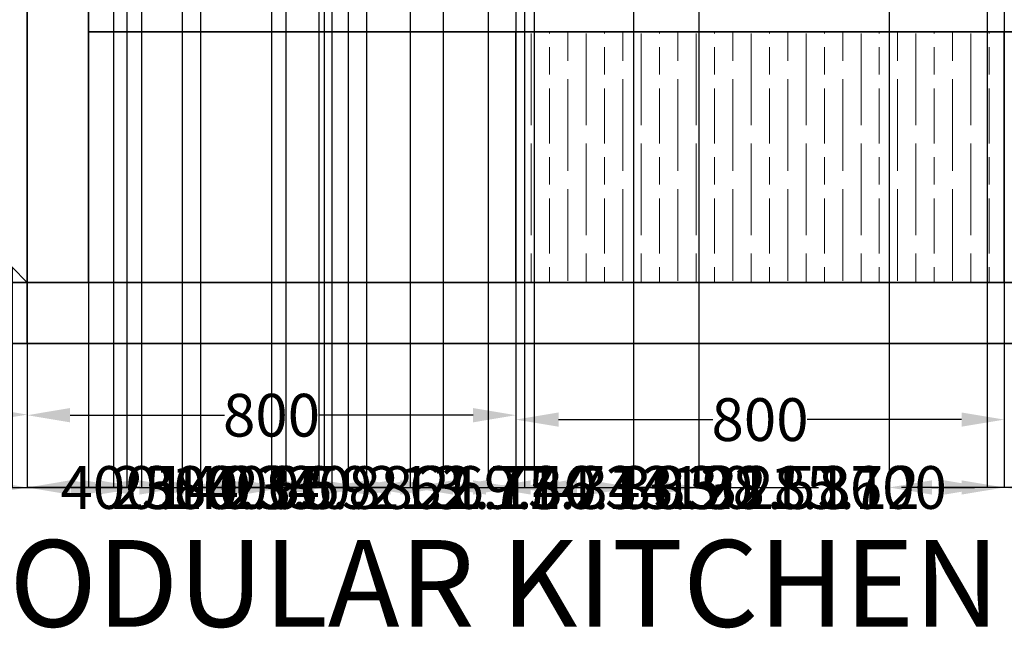
# Model space of a CAD drawing. Units: inches. Extents: x 600 to 5582, y -464 to 3142.
# Tile 2 of 9: x 1772 to 3385, y -464 to 532. Entities that reach past the tile are written whole.
import ezdxf

# ---------------------------------------------------------------- set-up
doc = ezdxf.new("R2010")
doc.units = ezdxf.units.IN
doc.header["$MEASUREMENT"] = 0
for name, color, linetype, lineweight in [('A-ANNO-DIMS', 2, 'Continuous', 18), ('A-ANNO-TEXT', 7, 'Continuous', 25), ('A-ELEV', 7, 'Continuous', 35), ('A-ELEV-PATT', 252, 'Continuous', 13)]:
    doc.layers.add(name, color=color, linetype=linetype, lineweight=lineweight)
doc.styles.get("Standard").update_dxf_attribs({"font": 'arial.ttf'})
doc.dimstyles.get("Standard").update_dxf_attribs({"dimtxt": 70, "dimasz": 70, "dimexe": 0.18, "dimexo": 0.0625, "dimgap": 0.09, "dimtad": 0, "dimtih": 1, "dimtoh": 1, "dimdec": 0, "dimzin": 0, "dimdsep": 46, "dimtxsty": 'Standard', "dimcen": 0.09, "dimadec": 0, "dimazin": 0, "dimtfac": 1, "dimtdec": 0, "dimtofl": 0, "dimtmove": 0, "dimatfit": 3, "dimfxl": 1, "dimtolj": 1, "dimtzin": 0, "dimarcsym": 0})

# ---------------------------------------------------------------- blocks, each defined once
blk = doc.blocks.new('*D10')
at = {"layer": 'A-ANNO-DIMS', "color": 0, "lineweight": -2, "transparency": 16777216}
for p, q in [((1384.7, 2.4), (1384.7, -113.9)), ((1784.7, 2.4), (1784.7, -113.9)), ((1454.7, -113.8), (1506, -113.8)), ((1714.7, -113.8), (1663.5, -113.8))]:
    blk.add_line(p, q, dxfattribs=at)
at = {"layer": 'A-ANNO-DIMS', "color": 0, "transparency": 16777216}
for points in [[(1454.7, -102.1), (1454.7, -125.4), (1384.7, -113.8)], [(1714.7, -102.1), (1714.7, -125.4), (1784.7, -113.8)]]:
    blk.add_solid(points, dxfattribs=at)
at = {"layer": 'Defpoints', "color": 0, "transparency": 16777216}
for p in [(1384.7, 2.4), (1784.7, 2.4), (1784.7, -113.8)]:
    blk.add_point(p, dxfattribs=at)
at = {"layer": 'A-ANNO-DIMS', "color": 0, "transparency": 16777216, "insert": (1584.7, -113.8), "char_height": 70, "attachment_point": 5}
blk.add_mtext('\\A1;400', dxfattribs=at)
blk = doc.blocks.new('*D11')
at = {"layer": 'A-ANNO-DIMS', "color": 0, "lineweight": -2, "transparency": 16777216}
for p, q in [((1784.7, 2.4), (1784.7, -115)), ((2584.7, 2.4), (2584.7, -115)), ((1854.7, -114.8), (2107.4, -114.8)), ((2514.7, -114.8), (2262.1, -114.8))]:
    blk.add_line(p, q, dxfattribs=at)
at = {"layer": 'A-ANNO-DIMS', "color": 0, "transparency": 16777216}
for points in [[(1854.7, -103.1), (1854.7, -126.5), (1784.7, -114.8)], [(2514.7, -103.1), (2514.7, -126.5), (2584.7, -114.8)]]:
    blk.add_solid(points, dxfattribs=at)
at = {"layer": 'Defpoints', "color": 0, "transparency": 16777216}
for p in [(1784.7, 2.4), (2584.7, 2.4), (2584.7, -114.8)]:
    blk.add_point(p, dxfattribs=at)
at = {"layer": 'A-ANNO-DIMS', "color": 0, "transparency": 16777216, "insert": (2184.7, -114.8), "char_height": 70, "attachment_point": 5}
blk.add_mtext('\\A1;800', dxfattribs=at)
blk = doc.blocks.new('*D12')
at = {"layer": 'A-ANNO-DIMS', "color": 0, "lineweight": -2, "transparency": 16777216}
for p, q in [((2584.7, 2.4), (2584.7, -122.1)), ((3384.7, 2.4), (3384.7, -122.1)), ((2654.7, -122), (2907.4, -122)), ((3314.7, -122), (3062.1, -122))]:
    blk.add_line(p, q, dxfattribs=at)
at = {"layer": 'A-ANNO-DIMS', "color": 0, "transparency": 16777216}
for points in [[(2654.7, -110.3), (2654.7, -133.6), (2584.7, -122)], [(3314.7, -110.3), (3314.7, -133.6), (3384.7, -122)]]:
    blk.add_solid(points, dxfattribs=at)
at = {"layer": 'Defpoints', "color": 0, "transparency": 16777216}
for p in [(2584.7, 2.4), (3384.7, 2.4), (3384.7, -122)]:
    blk.add_point(p, dxfattribs=at)
at = {"layer": 'A-ANNO-DIMS', "color": 0, "transparency": 16777216, "insert": (2984.7, -122), "char_height": 70, "attachment_point": 5}
blk.add_mtext('\\A1;800', dxfattribs=at)
blk = doc.blocks.new('*D21')
at = {"layer": 'A-ANNO-DIMS', "color": 0, "lineweight": -2, "transparency": 16777216}
for p, q in [((1384.7, 2.4), (1384.7, -233.3)), ((4984.7, 2.4), (4984.7, -233.3)), ((1454.7, -233.1), (3080.3, -233.1)), ((4914.7, -233.1), (3289.2, -233.1))]:
    blk.add_line(p, q, dxfattribs=at)
at = {"layer": 'A-ANNO-DIMS', "color": 0, "transparency": 16777216}
for points in [[(1454.7, -221.4), (1454.7, -244.7), (1384.7, -233.1)], [(4914.7, -221.4), (4914.7, -244.7), (4984.7, -233.1)]]:
    blk.add_solid(points, dxfattribs=at)
at = {"layer": 'Defpoints', "color": 0, "transparency": 16777216}
for p in [(1384.7, 2.4), (4984.7, 2.4), (4984.7, -233.1)]:
    blk.add_point(p, dxfattribs=at)
at = {"layer": 'A-ANNO-DIMS', "color": 0, "transparency": 16777216, "insert": (3184.7, -233.1), "char_height": 70, "attachment_point": 5}
blk.add_mtext('\\A1;3600', dxfattribs=at)
blk = doc.blocks.new('*D25')
at = {"layer": 'A-ANNO-DIMS', "color": 0, "lineweight": -2, "transparency": 16777216}
for p, q in [((2584.7, 1680.8), (2584.7, -233.3)), ((2615, 1655.8), (2615, -233.3)), ((2514.7, -233.1), (2444.7, -233.1)), ((2685, -233.1), (2755, -233.1))]:
    blk.add_line(p, q, dxfattribs=at)
at = {"layer": 'A-ANNO-DIMS', "color": 0, "transparency": 16777216}
for points in [[(2514.7, -221.4), (2514.7, -244.7), (2584.7, -233.1)], [(2685, -221.4), (2685, -244.7), (2615, -233.1)]]:
    blk.add_solid(points, dxfattribs=at)
at = {"layer": 'Defpoints', "color": 0, "transparency": 16777216}
for p in [(2584.7, 1680.8), (2615, 1655.8), (2615, -233.1)]:
    blk.add_point(p, dxfattribs=at)
at = {"layer": 'A-ANNO-DIMS', "color": 0, "transparency": 16777216, "insert": (2873.3, -233.1), "char_height": 70, "attachment_point": 5}
blk.add_mtext('\\A1;30.28', dxfattribs=at)
blk = doc.blocks.new('*D26')
at = {"layer": 'A-ANNO-DIMS', "color": 0, "lineweight": -2, "transparency": 16777216}
for p, q in [((3409.7, 1627.4), (3409.7, -233.3)), ((3384.7, 1602.4), (3384.7, -233.3)), ((3314.7, -233.1), (3244.7, -233.1)), ((3479.7, -233.1), (3549.7, -233.1))]:
    blk.add_line(p, q, dxfattribs=at)
at = {"layer": 'A-ANNO-DIMS', "color": 0, "transparency": 16777216}
for points in [[(3314.7, -221.4), (3314.7, -244.7), (3384.7, -233.1)], [(3479.7, -221.4), (3479.7, -244.7), (3409.7, -233.1)]]:
    blk.add_solid(points, dxfattribs=at)
at = {"layer": 'Defpoints', "color": 0, "transparency": 16777216}
for p in [(3409.7, 1627.4), (3384.7, 1602.4), (3409.7, -233.1)]:
    blk.add_point(p, dxfattribs=at)
at = {"layer": 'A-ANNO-DIMS', "color": 0, "transparency": 16777216, "insert": (3600.8, -233.1), "char_height": 70, "attachment_point": 5}
blk.add_mtext('\\A1;25', dxfattribs=at)
blk = doc.blocks.new('*D54')
at = {"layer": 'A-ANNO-DIMS', "color": 0, "lineweight": -2, "transparency": 16777216}
for p, q in [((1759.7, 127.4), (1759.7, -233.3)), ((1784.7, 102.4), (1784.7, -233.3)), ((1689.7, -233.1), (1619.7, -233.1)), ((1854.7, -233.1), (1924.7, -233.1))]:
    blk.add_line(p, q, dxfattribs=at)
at = {"layer": 'A-ANNO-DIMS', "color": 0, "transparency": 16777216}
for points in [[(1689.7, -221.4), (1689.7, -244.7), (1759.7, -233.1)], [(1854.7, -221.4), (1854.7, -244.7), (1784.7, -233.1)]]:
    blk.add_solid(points, dxfattribs=at)
at = {"layer": 'Defpoints', "color": 0, "transparency": 16777216}
for p in [(1759.7, 127.4), (1784.7, 102.4), (1784.7, -233.1)]:
    blk.add_point(p, dxfattribs=at)
at = {"layer": 'A-ANNO-DIMS', "color": 0, "transparency": 16777216, "insert": (1975.8, -233.1), "char_height": 70, "attachment_point": 5}
blk.add_mtext('\\A1;25', dxfattribs=at)
blk = doc.blocks.new('*D55')
at = {"layer": 'A-ANNO-DIMS', "color": 0, "lineweight": -2, "transparency": 16777216}
for p, q in [((1784.7, 102.4), (1784.7, -233.3)), ((1884.7, 102.4), (1884.7, -233.3)), ((1714.7, -233.1), (1644.7, -233.1)), ((1954.7, -233.1), (2024.7, -233.1))]:
    blk.add_line(p, q, dxfattribs=at)
at = {"layer": 'A-ANNO-DIMS', "color": 0, "transparency": 16777216}
for points in [[(1714.7, -221.4), (1714.7, -244.7), (1784.7, -233.1)], [(1954.7, -221.4), (1954.7, -244.7), (1884.7, -233.1)]]:
    blk.add_solid(points, dxfattribs=at)
at = {"layer": 'Defpoints', "color": 0, "transparency": 16777216}
for p in [(1784.7, 102.4), (1884.7, 102.4), (1884.7, -233.1)]:
    blk.add_point(p, dxfattribs=at)
at = {"layer": 'A-ANNO-DIMS', "color": 0, "transparency": 16777216, "insert": (2098.8, -233.1), "char_height": 70, "attachment_point": 5}
blk.add_mtext('\\A1;100', dxfattribs=at)
blk = doc.blocks.new('*D56')
at = {"layer": 'A-ANNO-DIMS', "color": 0, "lineweight": -2, "transparency": 16777216}
for p, q in [((1884.8, 512.4), (5220.4, 512.4)), ((5220.2, 442.4), (5220.2, 343.3)), ((5220.2, 172.4), (5220.2, 271.6)), ((1884.8, 102.4), (5220.4, 102.4))]:
    blk.add_line(p, q, dxfattribs=at)
at = {"layer": 'A-ANNO-DIMS', "color": 0, "transparency": 16777216}
for points in [[(5208.6, 442.4), (5231.9, 442.4), (5220.2, 512.4)], [(5208.6, 172.4), (5231.9, 172.4), (5220.2, 102.4)]]:
    blk.add_solid(points, dxfattribs=at)
at = {"layer": 'Defpoints', "color": 0, "transparency": 16777216}
for p in [(1884.7, 512.4), (5220.2, 512.4), (1884.7, 102.4)]:
    blk.add_point(p, dxfattribs=at)
at = {"layer": 'A-ANNO-DIMS', "color": 0, "transparency": 16777216, "insert": (5220.2, 307.4), "char_height": 70, "attachment_point": 5}
blk.add_mtext('\\A1;410', dxfattribs=at)
blk = doc.blocks.new('*D57')
at = {"layer": 'A-ANNO-DIMS', "color": 0, "lineweight": -2, "transparency": 16777216}
for p, q in [((5220.2, 622.4), (5220.2, 692.4)), ((5220.2, 692.4), (5290.2, 692.4)), ((1884.8, 552.4), (5220.4, 552.4)), ((1884.8, 512.4), (5220.4, 512.4)), ((5220.2, 442.4), (5220.2, 372.4))]:
    blk.add_line(p, q, dxfattribs=at)
at = {"layer": 'A-ANNO-DIMS', "color": 0, "transparency": 16777216}
for points in [[(5208.6, 622.4), (5231.9, 622.4), (5220.2, 552.4)], [(5208.6, 442.4), (5231.9, 442.4), (5220.2, 512.4)]]:
    blk.add_solid(points, dxfattribs=at)
at = {"layer": 'Defpoints', "color": 0, "transparency": 16777216}
for p in [(1884.7, 552.4), (5220.2, 552.4), (1884.7, 512.4)]:
    blk.add_point(p, dxfattribs=at)
at = {"layer": 'A-ANNO-DIMS', "color": 0, "transparency": 16777216, "insert": (5341.8, 692.4), "char_height": 70, "attachment_point": 5}
blk.add_mtext('\\A1;40', dxfattribs=at)
blk = doc.blocks.new('*D64')
at = {"layer": 'A-ANNO-DIMS', "color": 0, "lineweight": -2, "transparency": 16777216}
for p, q in [((3384.7, 1680.8), (3384.7, -233.3)), ((3356.6, 1655.8), (3356.6, -233.3)), ((3286.6, -233.1), (3216.6, -233.1)), ((3454.7, -233.1), (3524.7, -233.1))]:
    blk.add_line(p, q, dxfattribs=at)
at = {"layer": 'A-ANNO-DIMS', "color": 0, "transparency": 16777216}
for points in [[(3286.6, -221.4), (3286.6, -244.7), (3356.6, -233.1)], [(3454.7, -221.4), (3454.7, -244.7), (3384.7, -233.1)]]:
    blk.add_solid(points, dxfattribs=at)
at = {"layer": 'Defpoints', "color": 0, "transparency": 16777216}
for p in [(3384.7, 1680.8), (3356.6, 1655.8), (3384.7, -233.1)]:
    blk.add_point(p, dxfattribs=at)
at = {"layer": 'A-ANNO-DIMS', "color": 0, "transparency": 16777216, "insert": (3643.5, -233.1), "char_height": 70, "attachment_point": 5}
blk.add_mtext('\\A1;28.17', dxfattribs=at)
blk = doc.blocks.new('*D65')
at = {"layer": 'A-ANNO-DIMS', "color": 0, "lineweight": -2, "transparency": 16777216}
for p, q in [((1784.7, 2352.4), (1784.7, -233.3)), ((2184.7, 2352.4), (2184.7, -233.3)), ((1714.7, -233.1), (1644.7, -233.1)), ((2254.7, -233.1), (2324.7, -233.1))]:
    blk.add_line(p, q, dxfattribs=at)
at = {"layer": 'A-ANNO-DIMS', "color": 0, "transparency": 16777216}
for points in [[(1714.7, -221.4), (1714.7, -244.7), (1784.7, -233.1)], [(2254.7, -221.4), (2254.7, -244.7), (2184.7, -233.1)]]:
    blk.add_solid(points, dxfattribs=at)
at = {"layer": 'Defpoints', "color": 0, "transparency": 16777216}
for p in [(1784.7, 2352.4), (2184.7, 2352.4), (2184.7, -233.1)]:
    blk.add_point(p, dxfattribs=at)
at = {"layer": 'A-ANNO-DIMS', "color": 0, "transparency": 16777216, "insert": (1984.7, -233.1), "char_height": 70, "attachment_point": 5}
blk.add_mtext('\\A1;400.00', dxfattribs=at)
blk = doc.blocks.new('*D68')
at = {"layer": 'A-ANNO-DIMS', "color": 0, "lineweight": -2, "transparency": 16777216}
for p, q in [((2777.3, 1106.8), (2777.3, -233.3)), ((2584.7, 1002.4), (2584.7, -233.3)), ((2654.7, -233.1), (2707.3, -233.1)), ((2777.3, -233.1), (2847.3, -233.1))]:
    blk.add_line(p, q, dxfattribs=at)
at = {"layer": 'A-ANNO-DIMS', "color": 0, "transparency": 16777216}
for points in [[(2654.7, -221.4), (2654.7, -244.7), (2584.7, -233.1)], [(2707.3, -221.4), (2707.3, -244.7), (2777.3, -233.1)]]:
    blk.add_solid(points, dxfattribs=at)
at = {"layer": 'Defpoints', "color": 0, "transparency": 16777216}
for p in [(2777.3, 1106.8), (2584.7, 1002.4), (2777.3, -233.1)]:
    blk.add_point(p, dxfattribs=at)
at = {"layer": 'A-ANNO-DIMS', "color": 0, "transparency": 16777216, "insert": (2982.6, -233.1), "char_height": 70, "attachment_point": 5}
blk.add_mtext('\\A1;192.51', dxfattribs=at)
blk = doc.blocks.new('*D73')
at = {"layer": 'A-ANNO-DIMS', "color": 0, "lineweight": -2, "transparency": 16777216}
for p, q in [((2599.2, 1042.4), (2599.2, -233.3)), ((2584.7, 1002.4), (2584.7, -233.3)), ((2514.7, -233.1), (2444.7, -233.1)), ((2669.2, -233.1), (2739.2, -233.1))]:
    blk.add_line(p, q, dxfattribs=at)
at = {"layer": 'A-ANNO-DIMS', "color": 0, "transparency": 16777216}
for points in [[(2514.7, -221.4), (2514.7, -244.7), (2584.7, -233.1)], [(2669.2, -221.4), (2669.2, -244.7), (2599.2, -233.1)]]:
    blk.add_solid(points, dxfattribs=at)
at = {"layer": 'Defpoints', "color": 0, "transparency": 16777216}
for p in [(2599.2, 1042.4), (2584.7, 1002.4), (2599.2, -233.1)]:
    blk.add_point(p, dxfattribs=at)
at = {"layer": 'A-ANNO-DIMS', "color": 0, "transparency": 16777216, "insert": (2854, -233.1), "char_height": 70, "attachment_point": 5}
blk.add_mtext('\\A1;14.50', dxfattribs=at)
blk = doc.blocks.new('*D74')
at = {"layer": 'A-ANNO-DIMS', "color": 0, "lineweight": -2, "transparency": 16777216}
for p, q in [((2599.2, 1042.4), (2599.2, -233.3)), ((2884.4, 1042.4), (2884.4, -233.3)), ((2669.2, -233.1), (2814.4, -233.1)), ((2884.4, -233.1), (2954.4, -233.1))]:
    blk.add_line(p, q, dxfattribs=at)
at = {"layer": 'A-ANNO-DIMS', "color": 0, "transparency": 16777216}
for points in [[(2669.2, -221.4), (2669.2, -244.7), (2599.2, -233.1)], [(2814.4, -221.4), (2814.4, -244.7), (2884.4, -233.1)]]:
    blk.add_solid(points, dxfattribs=at)
at = {"layer": 'Defpoints', "color": 0, "transparency": 16777216}
for p in [(2599.2, 1042.4), (2884.4, 1042.4), (2884.4, -233.1)]:
    blk.add_point(p, dxfattribs=at)
at = {"layer": 'A-ANNO-DIMS', "color": 0, "transparency": 16777216, "insert": (3100, -233.1), "char_height": 70, "attachment_point": 5}
blk.add_mtext('\\A1;285.12', dxfattribs=at)
blk = doc.blocks.new('*D75')
at = {"layer": 'A-ANNO-DIMS', "color": 0, "lineweight": -2, "transparency": 16777216}
for p, q in [((2884.4, 1042.4), (2884.4, -233.3)), ((3196.2, 1042.4), (3196.2, -233.3)), ((2814.4, -233.1), (2744.4, -233.1)), ((3266.2, -233.1), (3336.2, -233.1))]:
    blk.add_line(p, q, dxfattribs=at)
at = {"layer": 'A-ANNO-DIMS', "color": 0, "transparency": 16777216}
for points in [[(2814.4, -221.4), (2814.4, -244.7), (2884.4, -233.1)], [(3266.2, -221.4), (3266.2, -244.7), (3196.2, -233.1)]]:
    blk.add_solid(points, dxfattribs=at)
at = {"layer": 'Defpoints', "color": 0, "transparency": 16777216}
for p in [(2884.4, 1042.4), (3196.2, 1042.4), (3196.2, -233.1)]:
    blk.add_point(p, dxfattribs=at)
at = {"layer": 'A-ANNO-DIMS', "color": 0, "transparency": 16777216, "insert": (3040.3, -233.1), "char_height": 70, "attachment_point": 5}
blk.add_mtext('\\A1;311.87', dxfattribs=at)
blk = doc.blocks.new('*D77')
at = {"layer": 'A-ANNO-DIMS', "color": 0, "lineweight": -2, "transparency": 16777216}
for p, q in [((1784.7, 1042.4), (1784.7, -233.3)), ((1925.7, 1042.4), (1925.7, -233.3)), ((1854.7, -233.1), (1855.7, -233.1)), ((1925.7, -233.1), (1995.7, -233.1))]:
    blk.add_line(p, q, dxfattribs=at)
at = {"layer": 'A-ANNO-DIMS', "color": 0, "transparency": 16777216}
for points in [[(1854.7, -221.4), (1854.7, -244.7), (1784.7, -233.1)], [(1855.7, -221.4), (1855.7, -244.7), (1925.7, -233.1)]]:
    blk.add_solid(points, dxfattribs=at)
at = {"layer": 'Defpoints', "color": 0, "transparency": 16777216}
for p in [(1784.7, 1042.4), (1925.7, 1042.4), (1925.7, -233.1)]:
    blk.add_point(p, dxfattribs=at)
at = {"layer": 'A-ANNO-DIMS', "color": 0, "transparency": 16777216, "insert": (2138.1, -233.1), "char_height": 70, "attachment_point": 5}
blk.add_mtext('\\A1;140.95', dxfattribs=at)
blk = doc.blocks.new('*D78')
at = {"layer": 'A-ANNO-DIMS', "color": 0, "lineweight": -2, "transparency": 16777216}
for p, q in [((1925.7, 1042.4), (1925.7, -233.3)), ((2310, 1042.4), (2310, -233.3)), ((1855.7, -233.1), (1785.7, -233.1)), ((2380, -233.1), (2450, -233.1))]:
    blk.add_line(p, q, dxfattribs=at)
at = {"layer": 'A-ANNO-DIMS', "color": 0, "transparency": 16777216}
for points in [[(1855.7, -221.4), (1855.7, -244.7), (1925.7, -233.1)], [(2380, -221.4), (2380, -244.7), (2310, -233.1)]]:
    blk.add_solid(points, dxfattribs=at)
at = {"layer": 'Defpoints', "color": 0, "transparency": 16777216}
for p in [(1925.7, 1042.4), (2310, 1042.4), (2310, -233.1)]:
    blk.add_point(p, dxfattribs=at)
at = {"layer": 'A-ANNO-DIMS', "color": 0, "transparency": 16777216, "insert": (2117.9, -233.1), "char_height": 70, "attachment_point": 5}
blk.add_mtext('\\A1;384.34', dxfattribs=at)
blk = doc.blocks.new('*D82')
at = {"layer": 'A-ANNO-DIMS', "color": 0, "lineweight": -2, "transparency": 16777216}
for p, q in [((1947.9, 1063.6), (1947.9, -233.3)), ((1971.5, 1063.3), (1971.5, -233.3)), ((1877.9, -233.1), (1807.9, -233.1)), ((2041.5, -233.1), (2111.5, -233.1))]:
    blk.add_line(p, q, dxfattribs=at)
at = {"layer": 'A-ANNO-DIMS', "color": 0, "transparency": 16777216}
for points in [[(1877.9, -221.4), (1877.9, -244.7), (1947.9, -233.1)], [(2041.5, -221.4), (2041.5, -244.7), (1971.5, -233.1)]]:
    blk.add_solid(points, dxfattribs=at)
at = {"layer": 'Defpoints', "color": 0, "transparency": 16777216}
for p in [(1947.9, 1063.7), (1971.5, 1063.4), (1971.5, -233.1)]:
    blk.add_point(p, dxfattribs=at)
at = {"layer": 'A-ANNO-DIMS', "color": 0, "transparency": 16777216, "insert": (2230.4, -233.1), "char_height": 70, "attachment_point": 5}
blk.add_mtext('\\A1;23.59', dxfattribs=at)
blk = doc.blocks.new('*D83')
at = {"layer": 'A-ANNO-DIMS', "color": 0, "lineweight": -2, "transparency": 16777216}
for p, q in [((1971.5, 1063.3), (1971.5, -233.3)), ((2038.4, 1063.3), (2038.4, -233.3)), ((1901.5, -233.1), (1831.5, -233.1)), ((2108.4, -233.1), (2178.4, -233.1))]:
    blk.add_line(p, q, dxfattribs=at)
at = {"layer": 'A-ANNO-DIMS', "color": 0, "transparency": 16777216}
for points in [[(1901.5, -221.4), (1901.5, -244.7), (1971.5, -233.1)], [(2108.4, -221.4), (2108.4, -244.7), (2038.4, -233.1)]]:
    blk.add_solid(points, dxfattribs=at)
at = {"layer": 'Defpoints', "color": 0, "transparency": 16777216}
for p in [(1971.5, 1063.4), (2038.4, 1063.4), (2038.4, -233.1)]:
    blk.add_point(p, dxfattribs=at)
at = {"layer": 'A-ANNO-DIMS', "color": 0, "transparency": 16777216, "insert": (2296.9, -233.1), "char_height": 70, "attachment_point": 5}
blk.add_mtext('\\A1;66.88', dxfattribs=at)
blk = doc.blocks.new('*D84')
at = {"layer": 'A-ANNO-DIMS', "color": 0, "lineweight": -2, "transparency": 16777216}
for p, q in [((2038.4, 1063.3), (2038.4, -233.3)), ((2068.6, 1063.3), (2068.6, -233.3)), ((1968.4, -233.1), (1898.4, -233.1)), ((2138.6, -233.1), (2208.6, -233.1))]:
    blk.add_line(p, q, dxfattribs=at)
at = {"layer": 'A-ANNO-DIMS', "color": 0, "transparency": 16777216}
for points in [[(1968.4, -221.4), (1968.4, -244.7), (2038.4, -233.1)], [(2138.6, -221.4), (2138.6, -244.7), (2068.6, -233.1)]]:
    blk.add_solid(points, dxfattribs=at)
at = {"layer": 'Defpoints', "color": 0, "transparency": 16777216}
for p in [(2038.4, 1063.4), (2068.6, 1063.4), (2068.6, -233.1)]:
    blk.add_point(p, dxfattribs=at)
at = {"layer": 'A-ANNO-DIMS', "color": 0, "transparency": 16777216, "insert": (2354, -233.1), "char_height": 70, "attachment_point": 5}
blk.add_mtext('\\A1;30.213', dxfattribs=at)
blk = doc.blocks.new('*D92')
at = {"layer": 'A-ANNO-DIMS', "color": 0, "lineweight": -2, "transparency": 16777216}
for p, q in [((2208.2, 1533.4), (2208.2, -233.3)), ((2271, 1533.4), (2271, -233.3)), ((2138.2, -233.1), (2068.2, -233.1)), ((2341, -233.1), (2411, -233.1))]:
    blk.add_line(p, q, dxfattribs=at)
at = {"layer": 'A-ANNO-DIMS', "color": 0, "transparency": 16777216}
for points in [[(2138.2, -221.4), (2138.2, -244.7), (2208.2, -233.1)], [(2341, -221.4), (2341, -244.7), (2271, -233.1)]]:
    blk.add_solid(points, dxfattribs=at)
at = {"layer": 'Defpoints', "color": 0, "transparency": 16777216}
for p in [(2208.2, 1533.5), (2271, 1533.5), (2271, -233.1)]:
    blk.add_point(p, dxfattribs=at)
at = {"layer": 'A-ANNO-DIMS', "color": 0, "transparency": 16777216, "insert": (2529.3, -233.1), "char_height": 70, "attachment_point": 5}
blk.add_mtext('\\A1;62.77', dxfattribs=at)
blk = doc.blocks.new('*D93')
at = {"layer": 'A-ANNO-DIMS', "color": 0, "lineweight": -2, "transparency": 16777216}
for p, q in [((2271, 1533.4), (2271, -233.3)), ((2340.4, 1533.4), (2340.4, -233.3)), ((2201, -233.1), (2131, -233.1)), ((2410.4, -233.1), (2480.4, -233.1))]:
    blk.add_line(p, q, dxfattribs=at)
at = {"layer": 'A-ANNO-DIMS', "color": 0, "transparency": 16777216}
for points in [[(2201, -221.4), (2201, -244.7), (2271, -233.1)], [(2410.4, -221.4), (2410.4, -244.7), (2340.4, -233.1)]]:
    blk.add_solid(points, dxfattribs=at)
at = {"layer": 'Defpoints', "color": 0, "transparency": 16777216}
for p in [(2271, 1533.5), (2340.4, 1533.5), (2340.4, -233.1)]:
    blk.add_point(p, dxfattribs=at)
at = {"layer": 'A-ANNO-DIMS', "color": 0, "transparency": 16777216, "insert": (2598.6, -233.1), "char_height": 70, "attachment_point": 5}
blk.add_mtext('\\A1;69.40', dxfattribs=at)
blk = doc.blocks.new('*D94')
at = {"layer": 'A-ANNO-DIMS', "color": 0, "lineweight": -2, "transparency": 16777216}
for p, q in [((2340.4, 1533.4), (2340.4, -233.3)), ((2411.7, 1533.4), (2411.7, -233.3)), ((2270.4, -233.1), (2200.4, -233.1)), ((2481.7, -233.1), (2551.7, -233.1))]:
    blk.add_line(p, q, dxfattribs=at)
at = {"layer": 'A-ANNO-DIMS', "color": 0, "transparency": 16777216}
for points in [[(2270.4, -221.4), (2270.4, -244.7), (2340.4, -233.1)], [(2481.7, -221.4), (2481.7, -244.7), (2411.7, -233.1)]]:
    blk.add_solid(points, dxfattribs=at)
at = {"layer": 'Defpoints', "color": 0, "transparency": 16777216}
for p in [(2340.4, 1533.5), (2411.7, 1533.5), (2411.7, -233.1)]:
    blk.add_point(p, dxfattribs=at)
at = {"layer": 'A-ANNO-DIMS', "color": 0, "transparency": 16777216, "insert": (2669.5, -233.1), "char_height": 70, "attachment_point": 5}
blk.add_mtext('\\A1;71.34', dxfattribs=at)
blk = doc.blocks.new('*D95')
at = {"layer": 'A-ANNO-DIMS', "color": 0, "lineweight": -2, "transparency": 16777216}
for p, q in [((2411.7, 1533.4), (2411.7, -233.3)), ((2465.8, 1533.4), (2465.8, -233.3)), ((2341.7, -233.1), (2271.7, -233.1)), ((2535.8, -233.1), (2605.8, -233.1))]:
    blk.add_line(p, q, dxfattribs=at)
at = {"layer": 'A-ANNO-DIMS', "color": 0, "transparency": 16777216}
for points in [[(2341.7, -221.4), (2341.7, -244.7), (2411.7, -233.1)], [(2535.8, -221.4), (2535.8, -244.7), (2465.8, -233.1)]]:
    blk.add_solid(points, dxfattribs=at)
at = {"layer": 'Defpoints', "color": 0, "transparency": 16777216}
for p in [(2411.7, 1533.5), (2465.8, 1533.5), (2465.8, -233.1)]:
    blk.add_point(p, dxfattribs=at)
at = {"layer": 'A-ANNO-DIMS', "color": 0, "transparency": 16777216, "insert": (2724, -233.1), "char_height": 70, "attachment_point": 5}
blk.add_mtext('\\A1;54.13', dxfattribs=at)
blk = doc.blocks.new('*D96')
at = {"layer": 'A-ANNO-DIMS', "color": 0, "lineweight": -2, "transparency": 16777216}
for p, q in [((2465.8, 1533.4), (2465.8, -233.3)), ((2539.2, 1533.4), (2539.2, -233.3)), ((2395.8, -233.1), (2325.8, -233.1)), ((2609.2, -233.1), (2679.2, -233.1))]:
    blk.add_line(p, q, dxfattribs=at)
at = {"layer": 'A-ANNO-DIMS', "color": 0, "transparency": 16777216}
for points in [[(2395.8, -221.4), (2395.8, -244.7), (2465.8, -233.1)], [(2609.2, -221.4), (2609.2, -244.7), (2539.2, -233.1)]]:
    blk.add_solid(points, dxfattribs=at)
at = {"layer": 'Defpoints', "color": 0, "transparency": 16777216}
for p in [(2465.8, 1533.5), (2539.2, 1533.5), (2539.2, -233.1)]:
    blk.add_point(p, dxfattribs=at)
at = {"layer": 'A-ANNO-DIMS', "color": 0, "transparency": 16777216, "insert": (2797.1, -233.1), "char_height": 70, "attachment_point": 5}
blk.add_mtext('\\A1;73.33', dxfattribs=at)
blk = doc.blocks.new('*D100')
at = {"layer": 'A-ANNO-DIMS', "color": 0, "lineweight": -2, "transparency": 16777216}
for p, q in [((2262.3, 1439.7), (2262.3, -233.3)), ((2283.5, 1439.7), (2283.5, -233.3)), ((2192.3, -233.1), (2122.3, -233.1)), ((2353.5, -233.1), (2423.5, -233.1))]:
    blk.add_line(p, q, dxfattribs=at)
at = {"layer": 'A-ANNO-DIMS', "color": 0, "transparency": 16777216}
for points in [[(2192.3, -221.4), (2192.3, -244.7), (2262.3, -233.1)], [(2353.5, -221.4), (2353.5, -244.7), (2283.5, -233.1)]]:
    blk.add_solid(points, dxfattribs=at)
at = {"layer": 'Defpoints', "color": 0, "transparency": 16777216}
for p in [(2262.3, 1439.7), (2283.5, 1439.7), (2283.5, -233.1)]:
    blk.add_point(p, dxfattribs=at)
at = {"layer": 'A-ANNO-DIMS', "color": 0, "transparency": 16777216, "insert": (2569.4, -233.1), "char_height": 70, "attachment_point": 5}
blk.add_mtext('\\A1;21.136', dxfattribs=at)

msp = doc.modelspace()

# ---------------------------------------------------------------- hatches: boundary and pattern name
at = {"layer": 'A-ELEV-PATT'}
h = msp.add_hatch(dxfattribs=at)
h.set_pattern_fill('GOST_WOOD', color=256, scale=15)
h.set_pattern_definition([(90, (0, 0), (90, -6e-15), [150, -30]), (90, (30, -30), (90, -6e-15), [90, -22.5, 45, -22.5]), (90, (60, -75), (90, -6e-15), [150, -30])])
h.paths.add_polyline_path([(4959.7485, 2752.4212), (1409.7485, 2752.4212), (1409.7485, 2352.4212), (1784.7485, 2352.4212), (4959.7485, 2352.4212)])
h.paths.add_polyline_path([(3384.7485, 1002.4212), (2584.7485, 1002.4212), (2584.7485, 777.4212), (3384.7485, 777.4212)])
h.paths.add_polyline_path([(3384.7485, 777.4212), (2584.7485, 777.4212), (2584.7485, 552.4212), (3384.7485, 552.4212)])
h.paths.add_polyline_path([(3384.7485, 512.4212), (2584.7485, 512.4212), (2584.7485, 102.4212), (3384.7485, 102.4212)])
h = msp.add_hatch(dxfattribs=at)
h.set_pattern_fill('CROSS', color=256, scale=100)
h.paths.add_polyline_path([(1759.7485, 2327.4212), (1409.7485, 2327.4212), (1409.7485, 1967.4212), (1759.7485, 1967.4212)])
h.paths.add_polyline_path([(1759.7485, 1952.4212), (1409.7485, 1952.4212), (1409.7485, 1567.4212), (1759.7485, 1567.4212)])
h.paths.add_polyline_path([(1759.7485, 1552.4212), (1409.7485, 1552.4212), (1409.7485, 1167.4212), (1759.7485, 1167.4212)])
h.paths.add_polyline_path([(1759.7485, 1152.4212), (1409.7485, 1152.4212), (1409.7485, 767.4212), (1759.7485, 767.4212)])
h.paths.add_polyline_path([(1759.7485, 752.4212), (1409.7485, 752.4212), (1409.7485, 367.4212), (1759.7485, 367.4212)])
h.paths.add_polyline_path([(1759.7485, 352.4212), (1409.7485, 352.4212), (1409.7485, 142.4212), (1759.7485, 142.4212)])
h.paths.add_polyline_path([(3759.7485, 1977.4212), (3409.7485, 1977.4212), (3409.7485, 1627.4212), (3759.7485, 1627.4212)])
h.paths.add_polyline_path([(3714.7508, 1954.858, -1), (3750.8891, 1954.858, -1)], flags=16)
h.paths.add_polyline_path([(3759.7485, 2327.4212), (3409.7485, 2327.4212), (3409.7485, 2002.4212), (3759.7485, 2002.4212)])
h.paths.add_polyline_path([(4159.7485, 2327.4212), (3809.7485, 2327.4212), (3809.7485, 2002.4212), (4159.7485, 2002.4212)])
h.paths.add_polyline_path([(4159.7485, 1977.4212), (3809.7485, 1977.4212), (3813.5467, 1954.858, -1), (3849.685, 1954.858, -1), (3813.5467, 1954.858), (3809.7485, 1627.4212), (4159.7485, 1627.4212)])
h.paths.add_polyline_path([(4559.7485, 2327.4212), (4184.7485, 2327.4212), (4184.7485, 2002.4212), (4559.7485, 2002.4212)])
h.paths.add_polyline_path([(4559.7485, 1977.4212), (4184.7485, 1977.4212), (4184.7485, 1627.4212), (4559.7485, 1627.4212)])
h.paths.add_polyline_path([(4517.0704, 1954.858, -1), (4553.2087, 1954.858, -1)], flags=16)
h.paths.add_polyline_path([(4959.7485, 2327.4212), (4609.7485, 2327.4212), (4609.7485, 2002.4212), (4959.7485, 2002.4212)])
h.paths.add_polyline_path([(4959.7485, 1977.4212), (4609.7485, 1977.4212), (4609.7485, 1627.4212), (4959.7485, 1627.4212)])
h.paths.add_polyline_path([(4619.5464, 1954.858, -1), (4655.6847, 1954.858, -1)], flags=16)

# ---------------------------------------------------------------- linework, layer by layer
at = {"layer": 'A-ELEV'}
for p, q in [((1884.7485, 102.4212), (1884.7485, 1002.4212)), ((4184.7485, 512.4212), (1884.7485, 512.4212)), ((2584.7485, 102.4212), (2584.7485, 512.4212)), ((3384.7485, 102.4212), (3384.7485, 512.4212)), ((4984.7485, 102.4212), (1384.7485, 102.4212))]:
    msp.add_line(p, q, dxfattribs=at)
for points in [[(4984.7485, 2.4212), (4984.7485, 2752.4212), (1384.7485, 2752.4212), (1384.7485, 2.4212)], [(1384.7485, 102.4212), (1409.7485, 127.4212), (1759.7485, 127.4212), (1784.7485, 102.4212)]]:
    msp.add_lwpolyline(points, close=True, dxfattribs=at)
msp.add_lwpolyline([(1784.7485, 2.4212), (1784.7485, 2352.4212), (1384.7485, 2352.4212), (1409.7485, 2327.4212), (1759.7485, 2327.4212), (1409.7485, 2327.4212), (1409.7485, 127.4212)], dxfattribs=at)

# ---------------------------------------------------------------- texts
at = {"layer": 'A-ANNO-TEXT'}
msp.add_text('MODULAR KITCHEN ELEVATION', height=141.903549, dxfattribs=at).set_placement((1598.0156, -460.987))

# ---------------------------------------------------------------- dimensions: what is measured, and where the dimension line sits
at = {"layer": 'A-ANNO-DIMS'}
for base, p1, p2, override, picture, middle in [((2184.7485, -233.0788), (1784.7485, 2352.4212), (2184.7485, 2352.4212), {"dimdec": 2, "dimlfac": 1, "dimrnd": 0, "dimzin": 0, "dimdsep": 46, "dimlunit": 2}, '*D65', (1984.7485, -233.0788)), ((2615.026, -233.0788), (2584.7485, 1680.8271), (2615.026, 1655.8271), {"dimdec": 2, "dimlfac": 1, "dimrnd": 0, "dimzin": 0, "dimdsep": 46, "dimlunit": 2}, '*D25', (2873.2709, -233.0788)), ((3384.7485, -233.0788), (3356.5781, 1655.8271), (3384.7485, 1680.8271), {"dimdec": 2, "dimlfac": 1, "dimrnd": 0, "dimzin": 0, "dimdsep": 46, "dimlunit": 2}, '*D64', (3643.5424, -233.0788)), ((3409.7485, -233.0788), (3384.7485, 1602.4212), (3409.7485, 1627.4212), {"dimdec": 0, "dimlfac": 1, "dimrnd": 0, "dimzin": 0, "dimdsep": 46, "dimlunit": 2}, '*D26', (3600.8344, -233.0788)), ((2270.9593, -233.0788), (2208.185, 1533.4874), (2270.9593, 1533.4874), {"dimdec": 2, "dimlfac": 1, "dimrnd": 0, "dimzin": 0, "dimdsep": 46, "dimlunit": 2}, '*D92', (2529.3474, -233.0788)), ((2340.3598, -233.0788), (2270.9593, 1533.4874), (2340.3598, 1533.4874), {"dimdec": 2, "dimlfac": 1, "dimrnd": 0, "dimzin": 0, "dimdsep": 46, "dimlunit": 2}, '*D93', (2598.6285, -233.0788)), ((2411.7034, -233.0788), (2340.3598, 1533.4874), (2411.7034, 1533.4874), {"dimdec": 2, "dimlfac": 1, "dimrnd": 0, "dimzin": 0, "dimdsep": 46, "dimlunit": 2}, '*D94', (2669.4707, -233.0788)), ((2465.8357, -233.0788), (2411.7034, 1533.4874), (2465.8357, 1533.4874), {"dimdec": 2, "dimlfac": 1, "dimrnd": 0, "dimzin": 0, "dimdsep": 46, "dimlunit": 2}, '*D95', (2724.0328, -233.0788)), ((2539.1643, -233.0788), (2465.8357, 1533.4874), (2539.1643, 1533.4874), {"dimdec": 2, "dimlfac": 1, "dimrnd": 0, "dimzin": 0, "dimdsep": 46, "dimlunit": 2}, '*D96', (2797.0749, -233.0788)), ((2283.4705, -233.0788), (2262.3346, 1439.718), (2283.4705, 1439.718), {"dimdec": 3, "dimlfac": 1, "dimrnd": 0, "dimzin": 0, "dimdsep": 46, "dimlunit": 2}, '*D100', (2569.4336, -233.0788)), ((2777.2556, -233.0788), (2584.7485, 1002.4212), (2777.2556, 1106.8415), {"dimdec": 2, "dimlfac": 1, "dimrnd": 0, "dimzin": 0, "dimdsep": 46, "dimlunit": 2}, '*D68', (2982.5946, -233.0788)), ((1971.5262, -233.0788), (1947.9344, 1063.682), (1971.5262, 1063.362), {"dimdec": 2, "dimlfac": 1, "dimrnd": 0, "dimzin": 0, "dimdsep": 46, "dimlunit": 2}, '*D82', (2230.3918, -233.0788)), ((2038.408, -233.0788), (1971.5262, 1063.362), (2038.408, 1063.362), {"dimdec": 2, "dimlfac": 1, "dimrnd": 0, "dimzin": 0, "dimdsep": 46, "dimlunit": 2}, '*D83', (2296.8677, -233.0788)), ((2068.6213, -233.0788), (2038.408, 1063.362), (2068.6213, 1063.362), {"dimdec": 3, "dimlfac": 1, "dimrnd": 0, "dimzin": 0, "dimdsep": 46, "dimlunit": 2}, '*D84', (2353.9875, -233.0788)), ((1925.6996, -233.0788), (1784.7485, 1042.4212), (1925.6996, 1042.4212), {"dimdec": 2, "dimlfac": 1, "dimrnd": 0, "dimzin": 0, "dimdsep": 46, "dimlunit": 2}, '*D77', (2138.0577, -233.0788)), ((2310.0444, -233.0788), (1925.6996, 1042.4212), (2310.0444, 1042.4212), {"dimdec": 2, "dimlfac": 1, "dimrnd": 0, "dimzin": 0, "dimdsep": 46, "dimlunit": 2}, '*D78', (2117.872, -233.0788)), ((2599.2497, -233.0788), (2584.7485, 1002.4212), (2599.2497, 1042.42), {"dimdec": 2, "dimlfac": 1, "dimrnd": 0, "dimzin": 0, "dimdsep": 46, "dimlunit": 2}, '*D73', (2854.0327, -233.0788)), ((2884.371, -233.0788), (2599.2497, 1042.42), (2884.371, 1042.4212), {"dimdec": 2, "dimlfac": 1, "dimrnd": 0, "dimzin": 0, "dimdsep": 46, "dimlunit": 2}, '*D74', (3099.9999, -233.0788)), ((3196.2381, -233.0788), (2884.371, 1042.4212), (3196.2381, 1042.4212), {"dimdec": 2, "dimlfac": 1, "dimrnd": 0, "dimzin": 0, "dimdsep": 46, "dimlunit": 2}, '*D75', (3040.3046, -233.0788)), ((1784.7485, -233.0788), (1759.7485, 127.4212), (1784.7485, 102.4212), {"dimdec": 0, "dimlfac": 1, "dimrnd": 0, "dimzin": 0, "dimdsep": 46, "dimlunit": 2}, '*D54', (1975.8344, -233.0788)), ((1884.7485, -233.0788), (1784.7485, 102.4212), (1884.7485, 102.4212), {"dimdec": 0, "dimlfac": 1, "dimrnd": 0, "dimzin": 0, "dimdsep": 46, "dimlunit": 2}, '*D55', (2098.7539, -233.0788)), ((1784.7485, -113.7624), (1384.7485, 2.4212), (1784.7485, 2.4212), {"dimclrd": 0, "dimclre": 0, "dimclrt": 0}, '*D10', (1584.7485, -113.7624)), ((4984.7485, -233.0788), (1384.7485, 2.4212), (4984.7485, 2.4212), {"dimdec": 0, "dimlfac": 1, "dimrnd": 0, "dimzin": 0, "dimdsep": 46, "dimlunit": 2}, '*D21', (3184.7485, -233.0788)), ((2584.7485, -114.8031), (1784.7485, 2.4212), (2584.7485, 2.4212), {"dimclrd": 0, "dimclre": 0, "dimclrt": 0}, '*D11', (2184.7485, -114.8031)), ((3384.7485, -121.967), (2584.7485, 2.4212), (3384.7485, 2.4212), {"dimclrd": 0, "dimclre": 0, "dimclrt": 0}, '*D12', (2984.7485, -121.967))]:
    dim = msp.add_linear_dim(base=base, p1=p1, p2=p2, dimstyle='Standard', override=override, dxfattribs=at)
    dim.commit()
    dim.dimension.update_dxf_attribs({"geometry": picture, "text_midpoint": middle})
for base, p1, p2, picture, middle in [((5220.2485, 552.4212), (1884.7485, 512.4212), (1884.7485, 552.4212), '*D57', (5341.7641, 692.4212)), ((5220.2485, 512.4212), (1884.7485, 102.4212), (1884.7485, 512.4212), '*D56', (5220.2485, 307.4212))]:
    dim = msp.add_linear_dim(base=base, p1=p1, p2=p2, angle=90, dimstyle='Standard', override={"dimdec": 0, "dimlfac": 1, "dimrnd": 0, "dimzin": 0, "dimdsep": 46, "dimlunit": 2}, dxfattribs=at)
    dim.commit()
    dim.dimension.update_dxf_attribs({"geometry": picture, "text_midpoint": middle})

doc.saveas('drawing.dxf')
